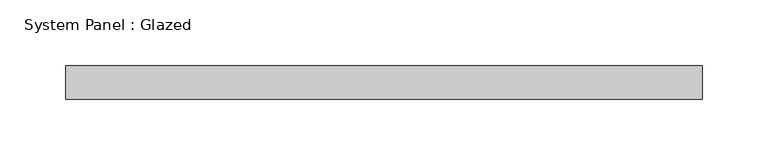
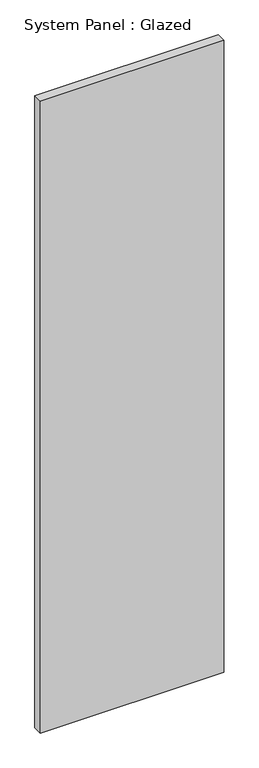
"""IFC4 building model written with IfcOpenShell, lengths in millimetres: plate geometry, System Panel : Glazed."""

from ifc_helpers import new_model, si_unit, origin, origin_with_axes, place, context, project, spatial, polyline, outline, extrude, source, transform, mapped, element, save


def system_panel_glazed_668e0709(model_context):
    return source(origin(), model_context, "Body", "SweptSolid", [
        extrude(outline(polyline([(241.3, 19.05), (-241.3, 19.05), (-241.3, 44.45), (241.3, 44.45), (241.3, 19.05)])), origin_with_axes(), (0.0, 0.0, 1.0), 1758.7876892),
    ])


if __name__ == "__main__":
    model = new_model("IFC4")
    model_context = context("Model", 3, world=origin())
    ifc_project = project(units=[si_unit("LENGTHUNIT", "METRE", prefix="MILLI")], contexts=[model_context])
    site = spatial("IfcSite", under=ifc_project)
    building = spatial("IfcBuilding", under=site)
    placement = place(None, origin())
    system_panel_glazed_shape = system_panel_glazed_668e0709(model_context)
    element("IfcPlate", 1, ObjectType="System Panel : Glazed", at=placement, inside=building, context=model_context, shape_type="MappedRepresentation", body=[
        mapped(system_panel_glazed_shape, transform((0.0, 0.0, 0.0), x_axis=(1.0, 0.0, 0.0), y_axis=(0.0, 1.0, 0.0), z_axis=(0.0, 0.0, 1.0))),
    ])
    save(model, "model.ifc")

# Revit data of these elements
# Type "System Panel : Glazed"
#   Construction Type Id = "GSP4R"
#   Analytic Construction = "1/8 in Pilkington single glazing"
#   Visual Light Transmittance = 0.9
#   Solar Heat Gain Coefficient = 0.86
#   Heat Transfer Coefficient (U) = 1.18115 BTU/(h·ft²·°F)
#   Define Thermal Properties by = 1
# Element 1 (IfcPlate, "System Panel : Glazed")
#   Materials on its faces: "Glass"
# Materials
#   "Glass": class "Glass", colour RGB 0 128 192, transparency 0.75, Description = "Soda Lime Glass", Cost = 0
